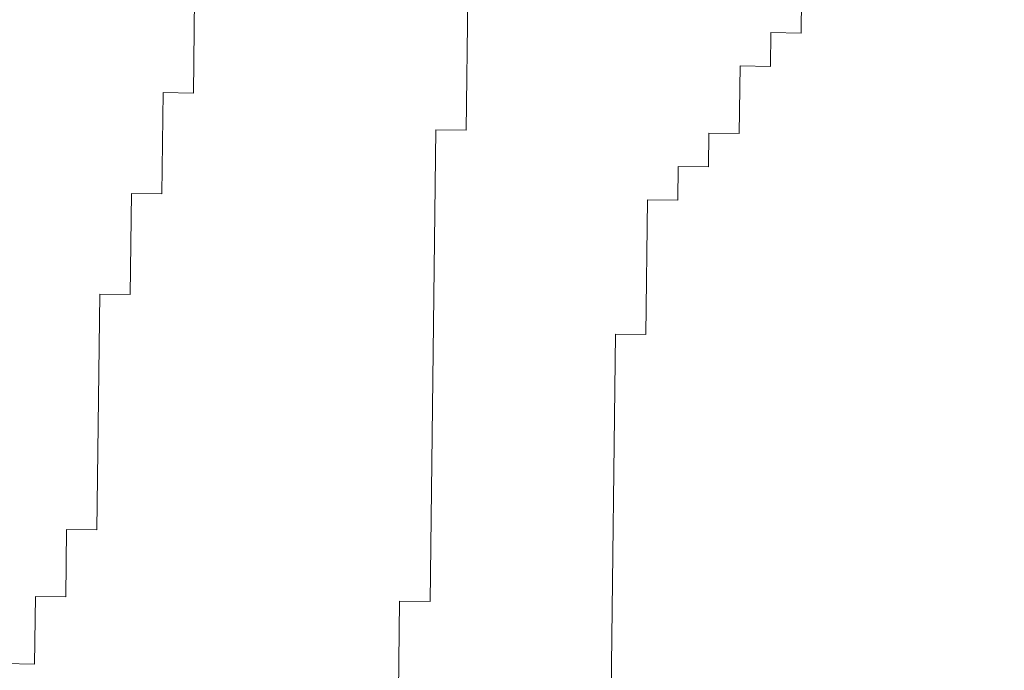
# Model space of a CAD drawing. Units: inches. Extents: x -466983 to 1020, y 324 to 318697.
# Tile 70 of 97: x 643.839 to 647.874, y 942.656 to 945.322. Entities that reach past the tile are written whole.
import ezdxf

# ---------------------------------------------------------------- set-up
doc = ezdxf.new("R2010")
doc.units = ezdxf.units.IN
doc.header["$MEASUREMENT"] = 0
doc.layers.add('A-FLOR-PATT', color=252, linetype='Continuous', lineweight=13)
doc.layers.add('A-FURN', color=8, linetype='Continuous', lineweight=18)

# ---------------------------------------------------------------- blocks, each defined once
blk = doc.blocks.new('L Shaped Sofa')
at = {"ltscale": 2}
for p, q in [((2414.2017, 741.2953), (2414.2417, 744.5701)), ((2415.8142, 743.2912), (2415.8234, 744.0469)), ((2418.5362, 743.2579), (2418.5424, 743.7617)), ((2418.5424, 743.7617), (2418.7692, 743.759)), ((2415.5443, 739.7672), (2415.5874, 743.294)), ((2415.5874, 743.294), (2415.8142, 743.2912)), ((2418.3033, 742.7569), (2418.3094, 743.2607)), ((2418.3094, 743.2607), (2418.5362, 743.2579)), ((2418.0549, 740.9963), (2418.0764, 742.7596)), ((2418.0764, 742.7596), (2418.3033, 742.7569)), ((2413.9626, 740.2904), (2413.9749, 741.2981)), ((2413.9749, 741.2981), (2414.2017, 741.2953)), ((2417.8188, 740.2433), (2417.828, 740.999)), ((2417.828, 740.999), (2418.0549, 740.9963)), ((2413.7327, 740.0413), (2413.7357, 740.2932)), ((2413.7357, 740.2932), (2413.9626, 740.2904)), ((2417.5827, 739.4903), (2417.592, 740.2461)), ((2417.592, 740.2461), (2417.8188, 740.2433)), ((2413.5028, 739.7921), (2413.5058, 740.044)), ((2413.5058, 740.044), (2413.7327, 740.0413)), ((2413.2698, 739.2911), (2413.2759, 739.7949)), ((2413.2759, 739.7949), (2413.5028, 739.7921)), ((2415.2897, 737.5028), (2415.3174, 739.77)), ((2415.3174, 739.77), (2415.5443, 739.7672)), ((2417.3467, 738.7374), (2417.3559, 739.4931)), ((2417.3559, 739.4931), (2417.5827, 739.4903)), ((2413.0398, 739.0419), (2413.0429, 739.2938)), ((2413.0429, 739.2938), (2413.2698, 739.2911)), ((2412.8069, 738.5409), (2412.813, 739.0447)), ((2412.813, 739.0447), (2413.0398, 739.0419))]:
    blk.add_line(p, q, dxfattribs=at)

msp = doc.modelspace()

# ---------------------------------------------------------------- hatches: boundary and pattern name
at = {"layer": 'A-FLOR-PATT', "transparency": 33554572}
h = msp.add_hatch(dxfattribs=at)
h.set_pattern_fill('ANSI37', color=256, scale=30)
h.set_pattern_definition([(45, (-1212.4137, -290.035), (-2.6516504, 2.6516504), []), (135, (-1212.4137, -290.035), (-2.6516504, -2.6516504), [])])
h.paths.add_polyline_path([(901.8057, 1075.9377), (900.6144, 1075.9377), (900.6144, 1065.3856), (899.391, 1065.3856), (898.0911, 1065.3856), (892.8356, 1058.7098, -0.258377), (892.1875, 1058.3509), (879.9848, 1058.3509, -0.20177), (879.4382, 1058.5808), (874.0812, 1065.3856), (872.7813, 1065.3856), (871.5579, 1065.3856), (871.5579, 1075.9377), (813.8057, 1075.9377), (813.8057, 1044.7922), (832.3947, 1044.7922, -0.394795), (848.6602, 1028.5356), (848.6602, 1009.9377), (901.8057, 1009.9377), (901.8057, 1015.9377), (901.3057, 1015.9377), (871.3057, 1015.9377), (871.3057, 1017.2502), (871.3344, 1017.2502, -0.401453), (901.3057, 1045.9377), (901.8057, 1045.9377)])
edge = h.paths.add_edge_path(flags=16)
edge.add_line((847.7731, 1068.9486), (847.7731, 1073.7088))
edge.add_arc((849.2269, 1073.7088), 1.4538, 90, 180, ccw=False)
edge.add_line((849.2269, 1075.1627), (864.4921, 1075.1627))
edge.add_arc((864.4921, 1073.7088), 1.4538, 0, 90, ccw=False)
edge.add_line((865.9459, 1073.7088), (865.9459, 1069.0035))
edge.add_arc((832.6447, 1068.9761), 33.3012, -20.61234, 0.04725, ccw=False)
edge.add_ellipse((856.8595, 1058.48), major_axis=(0, 10.2131), ratio=0.6859192, start_angle=100.00884, end_angle=259.99116, ccw=False)
edge.add_arc((881.0742, 1068.9761), 33.3012, 180.04725, 200.61234, ccw=False)
h.paths.add_polyline_path([(853.1456, 1066.4815), (853.1456, 1066.4534), (853.1463, 1066.4534, 0.433107), (852.9166, 1066.6849), (852.9166, 1066.4534), (853.1456, 1066.4534), (853.1456, 1066.4815), (853.088, 1066.6122, 0.697939), (852.6995, 1066.4534), (852.7003, 1066.4534), (852.7003, 1066.4815), (852.9166, 1067.0012), (852.9166, 1066.6849, -0.396254)], flags=0)
h.paths.add_polyline_path([(861.0187, 1066.4815), (861.0187, 1066.4534), (861.0194, 1066.4534, 0.416404), (860.8024, 1066.6849), (860.8024, 1066.4534), (861.0187, 1066.4534), (861.0187, 1066.4815), (860.9672, 1066.6053, 0.713344), (860.5726, 1066.4534), (860.5734, 1066.4534), (860.5734, 1066.4815), (860.8024, 1067.0012), (860.8024, 1066.6849, -0.379973)], flags=0)
edge = h.paths.add_edge_path(flags=0)
edge.add_spline(control_points=[(861.1298, 1065.7855), (861.4661, 1065.2478), (861.6134, 1065.0161), (861.9833, 1064.3736), (862.1924, 1063.9443), (862.5614, 1063.0391), (862.7212, 1062.5633), (862.9865, 1061.5781), (863.092, 1061.0689), (863.2452, 1060.031), (863.293, 1059.5025), (863.3295, 1058.4409), (863.3181, 1057.9078), (863.2366, 1056.8518), (863.1664, 1056.3289), (862.9695, 1055.308), (862.8427, 1054.8099), (862.5365, 1053.8522), (862.3571, 1053.3927), (861.9514, 1052.5249), (861.7251, 1052.1166), (861.233, 1051.3622), (860.9672, 1051.0162), (860.4048, 1050.3949), (860.1082, 1050.1197), (859.4937, 1049.6461), (859.1758, 1049.4476), (858.5276, 1049.1299), (858.1973, 1049.0107), (857.5315, 1048.8518), (857.1959, 1048.8121), (856.5249, 1048.812), (856.1894, 1048.8515), (855.5236, 1049.0101), (855.1933, 1049.1291), (854.545, 1049.4465), (854.2271, 1049.6449), (853.6124, 1050.1183), (853.3158, 1050.3933), (852.7533, 1051.0143), (852.4874, 1051.3602), (851.9952, 1052.1144), (851.7688, 1052.5225), (851.3629, 1053.3902), (851.1834, 1053.8496), (850.877, 1054.8071), (850.7501, 1055.3051), (850.553, 1056.326), (850.4827, 1056.8488), (850.401, 1057.9048), (850.3895, 1058.4379), (850.4257, 1059.4995), (850.4734, 1060.0281), (850.6265, 1061.066), (850.7318, 1061.5753), (850.9969, 1062.5605), (851.1567, 1063.0365), (851.5254, 1063.9418), (851.7345, 1064.3712), (852.1056, 1065.0164), (852.2544, 1065.2503), (852.6082, 1065.7335)], knot_values=[3.915332, 3.915332, 3.915332, 3.915332, 4.013468, 4.013468, 4.175532, 4.175532, 4.337596, 4.337596, 4.49966, 4.49966, 4.661724, 4.661724, 4.823788, 4.823788, 4.985852, 4.985852, 5.147916, 5.147916, 5.30998, 5.30998, 5.472044, 5.472044, 5.634109, 5.634109, 5.796173, 5.796173, 5.958237, 5.958237, 6.120301, 6.120301, 6.282365, 6.282365, 6.444429, 6.444429, 6.606493, 6.606493, 6.768557, 6.768557, 6.930621, 6.930621, 7.092685, 7.092685, 7.254749, 7.254749, 7.416813, 7.416813, 7.578878, 7.578878, 7.740942, 7.740942, 7.903006, 7.903006, 8.06507, 8.06507, 8.227134, 8.227134, 8.389198, 8.389198, 8.551262, 8.551262, 8.65037, 8.65037, 8.65037, 8.65037], degree=3, periodic=0)
edge.add_line((852.6421, 1065.7855), (861.1298, 1065.7855))
edge = h.paths.add_edge_path(flags=0)
edge.add_ellipse((856.8496, 1057.7432), major_axis=(0, 7.7921), ratio=0.687861, start_angle=0, end_angle=360)
h.paths.add_polyline_path([(848.8634, 1069.3891), (848.8634, 1073.9605, -0.414214), (849.9538, 1075.0508), (863.7652, 1075.0508, -0.414214), (864.8555, 1073.9605), (864.8555, 1069.3891, -0.388936), (864.5237, 1069.027, -0.043561), (849.1953, 1069.027, -0.388936)], flags=0)
h.paths.add_polyline_path([(853.1006, 1068.1122, -1), (852.6775, 1068.1122, -1)], flags=0)
edge = h.paths.add_edge_path(flags=0)
edge.add_ellipse((856.8595, 1057.3378), major_axis=(0, 2.207), ratio=0.657164, start_angle=0, end_angle=360)
h.paths.add_polyline_path([(861.0415, 1068.1122, -1), (860.6184, 1068.1122, -1)], flags=0)
edge = h.paths.add_edge_path()
edge.add_line((573.9537, 1057.3412), (573.9537, 1075.9377))
edge.add_line((573.9537, 1075.9377), (558.7308, 1075.9377))
edge.add_line((558.7308, 1075.9377), (558.7308, 1065.3856))
edge.add_line((558.7308, 1065.3856), (557.5074, 1065.3856))
edge.add_line((557.5074, 1065.3856), (556.2075, 1065.3856))
edge.add_line((556.2075, 1065.3856), (550.952, 1058.7098))
edge.add_arc((550.3039, 1059.1155), 0.7646, 270, 327.9483, ccw=False)
edge.add_line((550.3039, 1058.3509), (538.1012, 1058.3509))
edge.add_arc((538.1012, 1059.1155), 0.7646, 224.3704, 270, ccw=False)
edge.add_line((537.5546, 1058.5808), (532.1976, 1065.3856))
edge.add_line((532.1976, 1065.3856), (530.8977, 1065.3856))
edge.add_line((530.8977, 1065.3856), (529.6743, 1065.3856))
edge.add_line((529.6743, 1065.3856), (529.6743, 1075.9377))
edge.add_line((529.6743, 1075.9377), (520.8057, 1075.9377))
edge.add_line((520.8057, 1075.9377), (520.8057, 1045.9377))
edge.add_line((520.8057, 1045.9377), (521.3057, 1045.9377))
edge.add_arc((521.3057, 1015.9377), 30, 2.50749, 90, ccw=False)
edge.add_line((551.277, 1017.2502), (551.3057, 1017.2502))
edge.add_line((551.3057, 1017.2502), (551.3057, 1015.9377))
edge.add_line((551.3057, 1015.9377), (520.8057, 1015.9377))
edge.add_line((520.8057, 1015.9377), (520.8057, 1009.9377))
edge.add_line((520.8057, 1009.9377), (559.1913, 1010.4022))
edge.add_arc((559.1913, 1011.856), 1.4538, 180, 270, ccw=False)
edge.add_line((557.7375, 1011.856), (557.7375, 1016.5613))
edge.add_arc((591.0386, 1016.5888), 33.3012, 159.38766, 180.04725, ccw=False)
edge.add_ellipse((566.8239, 1027.0848), major_axis=(0, 10.2131), ratio=0.6859192, start_angle=280.00884, end_angle=439.99116, ccw=False)
edge.add_arc((542.6091, 1016.5888), 33.3012, 0.04725, 20.61234, ccw=False)
edge.add_line((575.9103, 1016.6162), (575.9103, 1011.856))
edge.add_arc((574.4565, 1011.856), 1.4538, -90, 0, ccw=False)
edge.add_line((574.4565, 1010.4022), (608.8057, 1009.9377))
edge.add_line((608.8057, 1009.9377), (608.8057, 1041.0857))
edge.add_line((608.8057, 1041.0857), (590.2179, 1041.0857))
edge.add_arc((590.775, 1057.9074), 16.8309, 181.92775, 268.10321, ccw=False)
edge = h.paths.add_edge_path()
edge.add_ellipse((494.2443, 583.6204), major_axis=(0, 10.2131), ratio=0.6859192, start_angle=280.00884, end_angle=439.99116, ccw=False)
edge.add_arc((470.0296, 573.1243), 33.3012, 0.04725, 20.61234, ccw=False)
edge.add_line((503.3307, 573.1518), (503.3307, 568.3916))
edge.add_arc((501.8769, 568.3916), 1.4538, -90, 0, ccw=False)
edge.add_line((501.8769, 566.9377), (539.8057, 566.9377))
edge.add_line((539.8057, 566.9377), (539.8057, 572.9377))
edge.add_line((539.8057, 572.9377), (539.3057, 572.9377))
edge.add_line((539.3057, 572.9377), (509.3057, 572.9377))
edge.add_line((509.3057, 572.9377), (509.3057, 574.2502))
edge.add_line((509.3057, 574.2502), (509.3344, 574.2502))
edge.add_arc((539.3057, 572.9377), 30, 90, 177.49251, ccw=False)
edge.add_line((539.3057, 602.9377), (539.8057, 602.9377))
edge.add_line((539.8057, 602.9377), (539.8057, 626.9377))
edge.add_line((539.8057, 626.9377), (531.7718, 626.9377))
edge.add_line((531.7718, 626.9377), (531.7718, 616.3856))
edge.add_line((531.7718, 616.3856), (530.5484, 616.3856))
edge.add_line((530.5484, 616.3856), (529.2485, 616.3856))
edge.add_line((529.2485, 616.3856), (523.7105, 609.3509))
edge.add_line((523.7105, 609.3509), (510.7766, 609.3509))
edge.add_line((510.7766, 609.3509), (505.2386, 616.3856))
edge.add_line((505.2386, 616.3856), (503.9387, 616.3856))
edge.add_line((503.9387, 616.3856), (502.7153, 616.3856))
edge.add_line((502.7153, 616.3856), (502.7153, 626.9377))
edge.add_line((502.7153, 626.9377), (481.6983, 626.9377))
edge.add_line((481.6983, 626.9377), (481.6983, 610.995))
edge.add_arc((467.2703, 611.4728), 14.4359, 271.92775, 358.10321, ccw=False)
edge.add_line((467.7559, 597.0451), (451.8057, 597.0451))
edge.add_line((451.8057, 597.0451), (451.8057, 584.4035))
edge.add_line((451.8057, 584.4035), (451.8057, 566.9377))
edge.add_line((451.8057, 566.9377), (486.6117, 566.9377))
edge.add_arc((486.6117, 568.3916), 1.4538, 180, 270, ccw=False)
edge.add_line((485.1579, 568.3916), (485.1579, 573.0969))
edge.add_arc((518.4591, 573.1243), 33.3012, 159.38766, 180.04725, ccw=False)
h.paths.add_polyline_path([(836.2609, 1020.7328), (879.8898, 1020.7328), (879.8898, 1039.3902), (836.2609, 1039.3902)], flags=25)
h.paths.add_polyline_path([(549.9851, 1036.7492), (593.614, 1036.7492), (593.614, 1055.4065), (549.9851, 1055.4065)], flags=24)
h.paths.add_polyline_path([(475.123, 595.5959), (518.752, 595.5959), (518.752, 614.2532), (475.123, 614.2532)], flags=24)
h = msp.add_hatch(dxfattribs=at)
h.set_pattern_fill('ANSI37', color=256, scale=20)
h.set_pattern_definition([(45, (-1212.4137, -290.035), (-1.767767, 1.767767), []), (135, (-1212.4137, -290.035), (-1.767767, -1.767767), [])])
h.paths.add_polyline_path([(809.8057, 870.9377), (809.8057, 888.1519), (806.9985, 888.1519), (802.6624, 888.1519), (789.3832, 888.1519), (786.2846, 888.1519, -0.414214), (785.4991, 888.9374), (785.4991, 900.1959), (785.4991, 908.4696, -0.414214), (786.8082, 909.7787, -0.414214), (785.4991, 911.0878), (785.4991, 929.1015, -0.414214), (786.8082, 930.4106, -0.414214), (785.4991, 931.7197), (785.4991, 931.9039, -0.414214), (784.19, 930.5948), (766.7223, 930.5948, -0.412359), (765.4132, 931.8956, -0.413741), (764.1145, 930.5782), (744.5781, 930.422, -0.416556), (743.7864, 931.2075), (743.7864, 933.5153), (742.2154, 933.5153), (742.2154, 952.024, -0.001344), (743.7864, 952.1998), (743.7864, 953.9377), (678.5915, 953.9377), (678.5915, 951.1305), (678.5915, 946.7945), (678.5915, 933.5153), (678.5915, 930.4166, -0.414214), (677.806, 929.6312), (666.5475, 929.6312), (658.2738, 929.6312, -0.414214), (656.9647, 930.9403, -0.414214), (655.6556, 929.6312), (637.6419, 929.6312, -0.414214), (636.3328, 930.9403, -0.414214), (635.0237, 929.6312), (634.8395, 929.6312, -0.414214), (636.1486, 928.322), (636.1486, 910.8544, -0.412359), (634.8478, 909.5452, -0.413741), (636.1653, 908.2466), (636.3214, 888.7102, -0.416556), (635.5359, 887.9184), (633.2281, 887.9184), (633.2281, 886.3475), (614.7194, 886.3475, -0.001344), (614.5436, 887.9184), (612.8057, 887.9184), (612.8057, 834.9377), (612.8057, 752.9377), (612.8057, 748.9377), (612.8057, 697.9377), (654.8057, 697.9377), (654.8057, 701.9377), (715.8057, 701.9377), (715.8057, 737.4353), (774.2918, 737.4353), (774.2918, 795.9377), (809.8057, 795.9377)])
h.paths.add_polyline_path([(679.2761, 849.5757, 0.102523), (682.1475, 849.2608, -0.080461), (694.5428, 849.7725, -0.283899), (694.4822, 849.0082, 0.136605), (694.4068, 848.8103, -0.030441), (694.5428, 846.8929), (694.5428, 842.6198), (694.5428, 838.3466, -0.028219), (694.4246, 836.5684), (694.425, 836.5684, 0.196187), (694.4456, 836.2708, -0.302897), (694.5428, 835.467, -0.080461), (682.1475, 835.9787, 0.102523), (679.2761, 835.6638, -0.58611), (678.6457, 836.0169), (678.6457, 849.2227, -0.58611)], flags=16)
h.paths.add_polyline_path([(679.5173, 848.6515, 0.699597), (679.476, 848.6342, 1.20716), (679.1935, 848.7422, 0.010621)], flags=0)
h.paths.add_polyline_path([(679.4923, 836.5608, -0.013798), (679.9178, 836.6594, -0.071703), (682.8533, 837.1434, -0.165743), (682.1665, 839.1006), (682.1665, 842.6094), (682.1665, 846.0603, -0.240616), (683.4733, 848.6767, -0.068263), (693.9295, 849.0082), (693.7875, 848.7083), (693.7875, 849.0228, 0.067332), (683.4733, 848.6767, 0.240616), (682.1665, 846.0603), (682.1665, 842.6094), (682.1665, 839.1006, 0.23459), (683.461, 836.5513, 0.068093), (693.7875, 836.1955), (693.7875, 836.5104), (693.9296, 836.2102, -0.077215), (682.2421, 836.7815, 0.086627), (679.5283, 836.5701, -0.628402), (679.5029, 836.5735), (679.5029, 836.6071, 0.910458)], flags=0)
h.paths.add_polyline_path([(679.476, 848.6364), (679.2069, 848.647), (679.2069, 836.5718, 0.913566), (679.3645, 836.5861), (679.476, 836.5824)], flags=0)
h.paths.add_polyline_path([(679.2761, 829.8604, 0.102523), (682.1475, 829.5455, -0.080461), (694.5428, 830.0572, -0.283899), (694.4822, 829.2929, 0.136605), (694.4068, 829.095, -0.030441), (694.5428, 827.1776), (694.5428, 822.9045), (694.5428, 818.6314, -0.028219), (694.4246, 816.8531), (694.425, 816.8532, 0.196187), (694.4456, 816.5555, -0.302897), (694.5428, 815.7517, -0.080461), (682.1475, 816.2635, 0.102523), (679.2761, 815.9485, -0.58611), (678.6457, 816.3016), (678.6457, 829.5074, -0.58611)], flags=16)
h.paths.add_polyline_path([(679.5173, 828.9362, 0.699597), (679.476, 828.9189, 1.20716), (679.1935, 829.0269, 0.010621)], flags=0)
h.paths.add_polyline_path([(679.4923, 816.8456, -0.013798), (679.9178, 816.9441, -0.071703), (682.8533, 817.4281, -0.165743), (682.1665, 819.3853), (682.1665, 822.8941), (682.1665, 826.345, -0.240616), (683.4733, 828.9614, -0.068263), (693.9295, 829.2929), (693.7875, 828.9931), (693.7875, 829.3076, 0.067332), (683.4733, 828.9614, 0.240616), (682.1665, 826.345), (682.1665, 822.8941), (682.1665, 819.3853, 0.23459), (683.461, 816.836, 0.068093), (693.7875, 816.4802), (693.7875, 816.7952), (693.9296, 816.4949, -0.077215), (682.2421, 817.0662, 0.086627), (679.5283, 816.8549, -0.628402), (679.5029, 816.8582), (679.5029, 816.8918, 0.910458)], flags=0)
h.paths.add_polyline_path([(679.476, 828.9211), (679.2069, 828.9317), (679.2069, 816.8565, 0.913566), (679.3645, 816.8708), (679.476, 816.8671)], flags=0)
h.paths.add_polyline_path([(679.2761, 810.1451, 0.102523), (682.1475, 809.8302, -0.080461), (694.5428, 810.342, -0.3023), (694.4466, 809.5394, 0.10023), (694.4058, 809.3878, -0.03057), (694.5428, 807.4623), (694.5428, 803.1892), (694.5428, 798.9161, -0.03057), (694.4058, 796.9906, 0.10023), (694.4466, 796.839, -0.3023), (694.5428, 796.0365, -0.080461), (682.1475, 796.5482, 0.102523), (679.2761, 796.2333, -0.58611), (678.6457, 796.5863), (678.6457, 809.7921, -0.58611)], flags=16)
h.paths.add_polyline_path([(679.5173, 809.2417, 0.699597), (679.476, 809.2244, 1.20716), (679.1935, 809.3324, 0.010621)], flags=0)
h.paths.add_polyline_path([(679.4923, 797.151, -0.013798), (679.9178, 797.2496, -0.071703), (682.8533, 797.7336, -0.165743), (682.1665, 799.6908), (682.1665, 803.1996), (682.1665, 806.6505, -0.239349), (683.461, 809.2577, -0.072465), (694.4468, 809.5405, 0.197932), (694.425, 809.2405), (693.7875, 809.2985), (693.7875, 809.6135, 0.068093), (683.461, 809.2577, 0.239349), (682.1665, 806.6505), (682.1665, 803.1996), (682.1665, 799.6908, 0.235854), (683.4733, 797.1323, 0.067332), (693.7875, 796.7861), (693.7875, 797.1006), (694.425, 797.1586, 0.197932), (694.4468, 796.8586, -0.080419), (682.1557, 797.3795, 0.083867), (679.5283, 797.1603, -0.628402), (679.5029, 797.1637), (679.5029, 797.1973, 0.910458)], flags=0)
h.paths.add_polyline_path([(679.2069, 809.2372), (679.2069, 797.162, 0.913566), (679.3645, 797.1763), (679.476, 797.1726), (679.476, 809.2266)], flags=0)
h.paths.add_polyline_path([(695.3643, 853.2989), (728.2231, 853.2989), (728.2231, 771.1519), (695.3643, 771.1519)], flags=16)
h.paths.add_polyline_path([(696.0215, 852.6417), (727.5659, 852.6417), (727.5659, 771.809), (696.0215, 771.809)], flags=0)
h.paths.add_polyline_path([(679.2761, 788.7869, 0.102523), (682.1475, 788.472, -0.080461), (694.5428, 788.9837, -0.3023), (694.4466, 788.1812, 0.10023), (694.4058, 788.0296, -0.03057), (694.5428, 786.1041), (694.5428, 781.831), (694.5428, 777.5578, -0.03057), (694.4058, 775.6323, 0.10023), (694.4466, 775.4808, -0.3023), (694.5428, 774.6782, -0.080461), (682.1475, 775.19, 0.102523), (679.2761, 774.875, -0.58611), (678.6457, 775.2281), (678.6457, 788.4339, -0.58611)], flags=16)
h.paths.add_polyline_path([(679.5173, 787.8834, 0.699597), (679.476, 787.8662, 1.20716), (679.1935, 787.9742, 0.010621)], flags=0)
h.paths.add_polyline_path([(679.4923, 775.7928, -0.013798), (679.9178, 775.8914, -0.071703), (682.8533, 776.3753, -0.165743), (682.1665, 778.3325), (682.1665, 781.8414), (682.1665, 785.2922, -0.239349), (683.461, 787.8995, -0.072465), (694.4468, 788.1823, 0.197932), (694.425, 787.8823), (693.7875, 787.9403), (693.7875, 788.2553, 0.068093), (683.461, 787.8995, 0.239349), (682.1665, 785.2922), (682.1665, 781.8414), (682.1665, 778.3325, 0.235854), (683.4733, 775.7741, 0.067332), (693.7875, 775.4279), (693.7875, 775.7424), (694.425, 775.8004, 0.197932), (694.4468, 775.5004, -0.080419), (682.1557, 776.0212, 0.083867), (679.5283, 775.8021, -0.628402), (679.5029, 775.8054), (679.5029, 775.8391, 0.910458)], flags=0)
h.paths.add_polyline_path([(679.2069, 787.8789), (679.2069, 775.8038, 0.913566), (679.3645, 775.818), (679.476, 775.8144), (679.476, 787.8684)], flags=0)
h.paths.add_polyline_path([(704.641, 854.1204, -0.080461), (705.1527, 866.5157, 0.102523), (704.8378, 869.3871, -0.58611), (705.1908, 870.0174), (718.3966, 870.0174, -0.58611), (718.7496, 869.3871, 0.102523), (718.4347, 866.5157, -0.080461), (718.9465, 854.1204, -0.3023), (718.1439, 854.2166, 0.10023), (717.9924, 854.2574, -0.03057), (716.0668, 854.1204), (711.7937, 854.1204), (707.5206, 854.1204, -0.03057), (705.5951, 854.2574, 0.10023), (705.4435, 854.2166, -0.3023)], flags=16)
h.paths.add_polyline_path([(717.8462, 869.1459, 0.699597), (717.8289, 869.1872, 1.20716), (717.9369, 869.4697, 0.010621)], flags=0)
h.paths.add_polyline_path([(705.4631, 854.2164, -0.080419), (705.984, 866.5074, 0.083867), (705.7648, 869.1349, -0.628402), (705.7682, 869.1603), (705.8018, 869.1603, 0.910458), (705.7555, 869.1709, -0.013798), (705.8541, 868.7454, -0.071703), (706.3381, 865.8099, -0.165743), (708.2953, 866.4967), (711.8041, 866.4967), (715.255, 866.4967, -0.239349), (717.8622, 865.2022, -0.072465), (718.145, 854.2164, 0.197932), (717.845, 854.2382), (717.903, 854.8757), (718.218, 854.8757, 0.068093), (717.8622, 865.2022, 0.239349), (715.255, 866.4967), (711.8041, 866.4967), (708.2953, 866.4967, 0.235854), (705.7368, 865.1898, 0.067332), (705.3906, 854.8757), (705.7051, 854.8757), (705.7631, 854.2382, 0.197932)], flags=16)
h.paths.add_polyline_path([(705.7665, 869.4563, 0.913566), (705.7808, 869.2987), (705.7771, 869.1872), (717.8311, 869.1872), (717.8417, 869.4563)], flags=0)
h.paths.add_polyline_path([(729.0446, 842.6198), (729.0446, 846.8929, -0.03057), (729.1817, 848.8184, 0.10023), (729.1408, 848.9699, -0.3023), (729.0446, 849.7725, -0.080461), (741.4399, 849.2608, 0.102523), (744.3113, 849.5757, -0.58611), (744.9417, 849.2227), (744.9417, 836.0169, -0.58611), (744.3113, 835.6638, 0.102523), (741.4399, 835.9787, -0.080461), (729.0446, 835.467, -0.3023), (729.1408, 836.2696, 0.10023), (729.1817, 836.4211, -0.03057), (729.0446, 838.3466)], flags=16)
h.paths.add_polyline_path([(744.1115, 836.5846, 1.20716), (744.3939, 836.4766, 0.010621), (744.0701, 836.5673, 0.699597)], flags=0)
h.paths.add_polyline_path([(729.1407, 836.2684, 0.197932), (729.1624, 836.5684), (729.7999, 836.5104), (729.7999, 836.1955, 0.068093), (740.1264, 836.5513, 0.239349), (741.4209, 839.1585), (741.4209, 842.6094), (741.4209, 846.1182, 0.235854), (740.1141, 848.6767, 0.067332), (729.7999, 849.0228), (729.7999, 848.7083), (729.1624, 848.6503, 0.197932), (729.1407, 848.9504, -0.080419), (741.4317, 848.4295, 0.083867), (744.0591, 848.6486, -0.628402), (744.0845, 848.6453), (744.0845, 848.6117, 0.910458), (744.0951, 848.6579, -0.013798), (743.6696, 848.5594, -0.071703), (740.7341, 848.0754, -0.165743), (741.4209, 846.1182), (741.4209, 842.6094), (741.4209, 839.1585, -0.239349), (740.1264, 836.5513, -0.072465)], flags=0)
h.paths.add_polyline_path([(729.0446, 830.0572, -0.080461), (741.4399, 829.5455, 0.102523), (744.3113, 829.8604, -0.58611), (744.9417, 829.5074), (744.9417, 816.3016, -0.58611), (744.3113, 815.9485, 0.102523), (741.4399, 816.2635, -0.080461), (729.0446, 815.7517, -0.3023), (729.1408, 816.5543, 0.10023), (729.1817, 816.7058, -0.03057), (729.0446, 818.6314), (729.0446, 822.9045), (729.0446, 827.1776, -0.03057), (729.1817, 829.1031, 0.10023), (729.1408, 829.2547, -0.3023)], flags=16)
h.paths.add_polyline_path([(744.1115, 816.8693, 1.20716), (744.3939, 816.7613, 0.010621), (744.0701, 816.852, 0.699597)], flags=0)
h.paths.add_polyline_path([(729.1407, 829.2351, -0.080419), (741.4317, 828.7142, 0.083867), (744.0591, 828.9334, -0.628402), (744.0845, 828.93), (744.0845, 828.8964, 0.910458), (744.0951, 828.9427, -0.013798), (743.6696, 828.8441, -0.071703), (740.7341, 828.3601, -0.165743), (741.4209, 826.4029), (741.4209, 822.8941), (741.4209, 819.4432, -0.239349), (740.1264, 816.836, -0.072465), (729.1407, 816.5531, 0.197932), (729.1624, 816.8532), (729.7999, 816.7952), (729.7999, 816.4802, 0.068093), (740.1264, 816.836, 0.239349), (741.4209, 819.4432), (741.4209, 822.8941), (741.4209, 826.4029, 0.235854), (740.1141, 828.9614, 0.067332), (729.7999, 829.3076), (729.7999, 828.9931), (729.1624, 828.9351, 0.197932)], flags=16)
h.paths.add_polyline_path([(729.0446, 810.342, -0.080461), (741.4399, 809.8302, 0.102523), (744.3113, 810.1451, -0.58611), (744.9417, 809.7921), (744.9417, 796.5863, -0.58611), (744.3113, 796.2333, 0.102523), (741.4399, 796.5482, -0.080461), (729.0446, 796.0365, -0.283899), (729.1052, 796.8007, 0.136605), (729.1806, 796.9987, -0.030441), (729.0446, 798.9161), (729.0446, 803.1892), (729.0446, 807.4623, -0.028219), (729.1628, 809.2406), (729.1624, 809.2405, 0.196187), (729.1418, 809.5382, -0.302897)], flags=16)
h.paths.add_polyline_path([(744.1115, 797.1748, 1.20716), (744.3939, 797.0668, 0.010621), (744.0701, 797.1575, 0.699597)], flags=0)
h.paths.add_polyline_path([(741.3453, 809.0275, 0.086627), (744.0591, 809.2388, -0.628402), (744.0845, 809.2355), (744.0845, 809.2019, 0.910458), (744.0951, 809.2481, -0.013798), (743.6696, 809.1496, -0.071703), (740.7341, 808.6656, -0.165743), (741.4209, 806.7084), (741.4209, 803.1996), (741.4209, 799.7487, -0.240616), (740.1141, 797.1323, -0.068263), (729.658, 796.8008), (729.7999, 797.1006), (729.7999, 796.7861, 0.067332), (740.1141, 797.1323, 0.240616), (741.4209, 799.7487), (741.4209, 803.1996), (741.4209, 806.7084, 0.23459), (740.1264, 809.2577, 0.068093), (729.7999, 809.6135), (729.7999, 809.2985), (729.6578, 809.5988, -0.077215)], flags=0)
h.paths.add_polyline_path([(704.641, 770.3304, -0.283899), (705.4053, 770.2697, 0.136605), (705.6032, 770.1944, -0.030441), (707.5206, 770.3304), (711.7937, 770.3304), (716.0668, 770.3304, -0.028219), (717.8451, 770.2122), (717.845, 770.2126, 0.196187), (718.1427, 770.2331, -0.302897), (718.9465, 770.3304, -0.080461), (718.4347, 757.9351, 0.102523), (718.7496, 755.0637, -0.58611), (718.3966, 754.4333), (705.1908, 754.4333, -0.58611), (704.8378, 755.0637, 0.102523), (705.1527, 757.9351, -0.080461)], flags=16)
h.paths.add_polyline_path([(705.762, 755.3048, 0.699597), (705.7793, 755.2635, 1.20716), (705.6713, 754.9811, 0.010621)], flags=0)
h.paths.add_polyline_path([(705.4053, 769.717), (705.7051, 769.5751), (705.3906, 769.5751, 0.067332), (705.7368, 759.2609, 0.240616), (708.3532, 757.954), (711.8041, 757.954), (715.3129, 757.954, 0.23459), (717.8622, 759.2485, 0.068093), (718.218, 769.5751), (717.903, 769.5751), (718.2033, 769.7172, -0.077215), (717.632, 758.0297, 0.086627), (717.8433, 755.3159, -0.628402), (717.84, 755.2904), (717.8064, 755.2904, 0.910458), (717.8526, 755.2799, -0.013798), (717.7541, 755.7053, -0.071703), (717.2701, 758.6409, -0.165743), (715.3129, 757.954), (711.8041, 757.954), (708.3532, 757.954, -0.240616), (705.7368, 759.2609, -0.068263)], flags=0)
h.paths.add_polyline_path([(729.0446, 788.9837, -0.080461), (741.4399, 788.472, 0.102523), (744.3113, 788.7869, -0.58611), (744.9417, 788.4339), (744.9417, 775.2281, -0.58611), (744.3113, 774.875, 0.102523), (741.4399, 775.19, -0.080461), (729.0446, 774.6782, -0.283899), (729.1052, 775.4425, 0.136605), (729.1806, 775.6405, -0.030441), (729.0446, 777.5578), (729.0446, 781.831), (729.0446, 786.1041, -0.028219), (729.1628, 787.8823), (729.1624, 787.8823, 0.196187), (729.1418, 788.1799, -0.302897)], flags=16)
h.paths.add_polyline_path([(744.1115, 775.8165, 1.20716), (744.3939, 775.7086, 0.010621), (744.0701, 775.7993, 0.699597)], flags=0)
h.paths.add_polyline_path([(741.3453, 787.6692, 0.086627), (744.0591, 787.8806, -0.628402), (744.0845, 787.8773), (744.0845, 787.8437, 0.910458), (744.0951, 787.8899, -0.013798), (743.6696, 787.7913, -0.071703), (740.7341, 787.3074, -0.165743), (741.4209, 785.3502), (741.4209, 781.8414), (741.4209, 778.3905, -0.240616), (740.1141, 775.7741, -0.068263), (729.658, 775.4425), (729.7999, 775.7424), (729.7999, 775.4279, 0.067332), (740.1141, 775.7741, 0.240616), (741.4209, 778.3905), (741.4209, 781.8414), (741.4209, 785.3502, 0.23459), (740.1264, 787.8995, 0.068093), (729.7999, 788.2553), (729.7999, 787.9403), (729.6578, 788.2405, -0.077215)], flags=0)
h.paths.add_polyline_path([(744.1115, 848.6364), (744.1115, 836.5824), (744.3805, 836.5718), (744.3805, 848.647, 0.913566), (744.2229, 848.6327)], flags=0)
h.paths.add_polyline_path([(744.2229, 828.9174), (744.1115, 828.9211), (744.1115, 816.8671), (744.3805, 816.8565), (744.3805, 828.9317, 0.913566)], flags=0)
h.paths.add_polyline_path([(717.8311, 755.2635), (705.7771, 755.2635), (705.7665, 754.9945), (717.8417, 754.9945, 0.913566), (717.8274, 755.1521)], flags=0)
h.paths.add_polyline_path([(744.2229, 809.2229), (744.1115, 809.2266), (744.1115, 797.1726), (744.3805, 797.162), (744.3805, 809.2372, 0.913566)], flags=0)
h.paths.add_polyline_path([(744.1115, 787.8684), (744.1115, 775.8144), (744.3805, 775.8038), (744.3805, 787.8789, 0.913566), (744.2229, 787.8647)], flags=0)
h.paths.add_polyline_path([(678.8774, 877.1228), (737.6127, 877.1228), (737.6127, 899.5116), (678.8774, 899.5116)], flags=24)

# ---------------------------------------------------------------- linework, layer by layer
at = {"layer": 'A-FURN', "ltscale": 2}
for p, q in [((645.6838, 946.1129), (645.6686, 944.8699)), ((645.6838, 946.1129), (645.6686, 944.8699)), ((645.6838, 946.1129), (645.6686, 944.8699)), ((645.6838, 946.1129), (645.6686, 944.8699)), ((645.6838, 946.1129), (645.6686, 944.8699)), ((645.6838, 946.1129), (645.6686, 944.8699)), ((647.045, 945.5437), (647.0416, 945.2675)), ((647.045, 945.5437), (647.0416, 945.2675)), ((647.045, 945.5437), (647.0416, 945.2675)), ((647.045, 945.5437), (647.0416, 945.2675)), ((647.045, 945.5437), (647.0416, 945.2675)), ((647.045, 945.5437), (647.0416, 945.2675)), ((644.5562, 945.436), (644.5511, 945.0217)), ((644.5562, 945.436), (644.5511, 945.0217)), ((644.5562, 945.436), (644.5511, 945.0217)), ((644.5562, 945.436), (644.5511, 945.0217)), ((644.5562, 945.436), (644.5511, 945.0217)), ((644.5562, 945.436), (644.5511, 945.0217)), ((646.9173, 945.2691), (646.9156, 945.131)), ((646.9173, 945.2691), (646.9156, 945.131)), ((646.9173, 945.2691), (646.9156, 945.131)), ((646.9173, 945.2691), (646.9156, 945.131)), ((646.9173, 945.2691), (646.9156, 945.131)), ((646.9173, 945.2691), (646.9156, 945.131)), ((647.0416, 945.2675), (646.9173, 945.2691)), ((647.0416, 945.2675), (646.9173, 945.2691)), ((647.0416, 945.2675), (646.9173, 945.2691)), ((647.0416, 945.2675), (646.9173, 945.2691)), ((647.0416, 945.2675), (646.9173, 945.2691)), ((647.0416, 945.2675), (646.9173, 945.2691)), ((646.7912, 945.1325), (646.7878, 944.8563)), ((646.7912, 945.1325), (646.7878, 944.8563)), ((646.7912, 945.1325), (646.7878, 944.8563)), ((646.7912, 945.1325), (646.7878, 944.8563)), ((646.7912, 945.1325), (646.7878, 944.8563)), ((646.7912, 945.1325), (646.7878, 944.8563)), ((646.9156, 945.131), (646.7912, 945.1325)), ((646.9156, 945.131), (646.7912, 945.1325)), ((646.9156, 945.131), (646.7912, 945.1325)), ((646.9156, 945.131), (646.7912, 945.1325)), ((646.9156, 945.131), (646.7912, 945.1325)), ((646.9156, 945.131), (646.7912, 945.1325)), ((644.4268, 945.0232), (644.4217, 944.6089)), ((644.4268, 945.0232), (644.4217, 944.6089)), ((644.4268, 945.0232), (644.4217, 944.6089)), ((644.4268, 945.0232), (644.4217, 944.6089)), ((644.4268, 945.0232), (644.4217, 944.6089)), ((644.4268, 945.0232), (644.4217, 944.6089)), ((644.5511, 945.0217), (644.4268, 945.0232)), ((644.5511, 945.0217), (644.4268, 945.0232)), ((644.5511, 945.0217), (644.4268, 945.0232)), ((644.5511, 945.0217), (644.4268, 945.0232)), ((644.5511, 945.0217), (644.4268, 945.0232)), ((644.5511, 945.0217), (644.4268, 945.0232)), ((645.5443, 944.8715), (645.5207, 942.938)), ((645.5443, 944.8715), (645.5207, 942.938)), ((645.5443, 944.8715), (645.5207, 942.938)), ((645.5443, 944.8715), (645.5207, 942.938)), ((645.5443, 944.8715), (645.5207, 942.938)), ((645.5443, 944.8715), (645.5207, 942.938)), ((645.6686, 944.8699), (645.5443, 944.8715)), ((645.6686, 944.8699), (645.5443, 944.8715)), ((645.6686, 944.8699), (645.5443, 944.8715)), ((645.6686, 944.8699), (645.5443, 944.8715)), ((645.6686, 944.8699), (645.5443, 944.8715)), ((645.6686, 944.8699), (645.5443, 944.8715)), ((646.6635, 944.8578), (646.6618, 944.7197)), ((646.6635, 944.8578), (646.6618, 944.7197)), ((646.6635, 944.8578), (646.6618, 944.7197)), ((646.6635, 944.8578), (646.6618, 944.7197)), ((646.6635, 944.8578), (646.6618, 944.7197)), ((646.6635, 944.8578), (646.6618, 944.7197)), ((646.7878, 944.8563), (646.6635, 944.8578)), ((646.7878, 944.8563), (646.6635, 944.8578)), ((646.7878, 944.8563), (646.6635, 944.8578)), ((646.7878, 944.8563), (646.6635, 944.8578)), ((646.7878, 944.8563), (646.6635, 944.8578)), ((646.7878, 944.8563), (646.6635, 944.8578)), ((646.5374, 944.7212), (646.5358, 944.5831)), ((646.5374, 944.7212), (646.5358, 944.5831)), ((646.5374, 944.7212), (646.5358, 944.5831)), ((646.5374, 944.7212), (646.5358, 944.5831)), ((646.5374, 944.7212), (646.5358, 944.5831)), ((646.5374, 944.7212), (646.5358, 944.5831)), ((646.6618, 944.7197), (646.5374, 944.7212)), ((646.6618, 944.7197), (646.5374, 944.7212)), ((646.6618, 944.7197), (646.5374, 944.7212)), ((646.6618, 944.7197), (646.5374, 944.7212)), ((646.6618, 944.7197), (646.5374, 944.7212)), ((646.6618, 944.7197), (646.5374, 944.7212)), ((644.2974, 944.6105), (644.2923, 944.1962)), ((644.2974, 944.6105), (644.2923, 944.1962)), ((644.2974, 944.6105), (644.2923, 944.1962)), ((644.2974, 944.6105), (644.2923, 944.1962)), ((644.2974, 944.6105), (644.2923, 944.1962)), ((644.2974, 944.6105), (644.2923, 944.1962)), ((644.4217, 944.6089), (644.2974, 944.6105)), ((644.4217, 944.6089), (644.2974, 944.6105)), ((644.4217, 944.6089), (644.2974, 944.6105)), ((644.4217, 944.6089), (644.2974, 944.6105)), ((644.4217, 944.6089), (644.2974, 944.6105)), ((644.4217, 944.6089), (644.2974, 944.6105)), ((646.4114, 944.5846), (646.4047, 944.0322)), ((646.4114, 944.5846), (646.4047, 944.0322)), ((646.4114, 944.5846), (646.4047, 944.0322)), ((646.4114, 944.5846), (646.4047, 944.0322)), ((646.4114, 944.5846), (646.4047, 944.0322)), ((646.4114, 944.5846), (646.4047, 944.0322)), ((646.5358, 944.5831), (646.4114, 944.5846)), ((646.5358, 944.5831), (646.4114, 944.5846)), ((646.5358, 944.5831), (646.4114, 944.5846)), ((646.5358, 944.5831), (646.4114, 944.5846)), ((646.5358, 944.5831), (646.4114, 944.5846)), ((646.5358, 944.5831), (646.4114, 944.5846)), ((644.1679, 944.1977), (644.1561, 943.231)), ((644.1679, 944.1977), (644.1561, 943.231)), ((644.1679, 944.1977), (644.1561, 943.231)), ((644.1679, 944.1977), (644.1561, 943.231)), ((644.1679, 944.1977), (644.1561, 943.231)), ((644.1679, 944.1977), (644.1561, 943.231)), ((644.2923, 944.1962), (644.1679, 944.1977)), ((644.2923, 944.1962), (644.1679, 944.1977)), ((644.2923, 944.1962), (644.1679, 944.1977)), ((644.2923, 944.1962), (644.1679, 944.1977)), ((644.2923, 944.1962), (644.1679, 944.1977)), ((644.2923, 944.1962), (644.1679, 944.1977)), ((646.2803, 944.0337), (646.2584, 942.2384)), ((646.2803, 944.0337), (646.2584, 942.2384)), ((646.2803, 944.0337), (646.2584, 942.2384)), ((646.2803, 944.0337), (646.2584, 942.2384)), ((646.2803, 944.0337), (646.2584, 942.2384)), ((646.2803, 944.0337), (646.2584, 942.2384)), ((646.4047, 944.0322), (646.2803, 944.0337)), ((646.4047, 944.0322), (646.2803, 944.0337)), ((646.4047, 944.0322), (646.2803, 944.0337)), ((646.4047, 944.0322), (646.2803, 944.0337)), ((646.4047, 944.0322), (646.2803, 944.0337)), ((646.4047, 944.0322), (646.2803, 944.0337)), ((644.0318, 943.2325), (644.0284, 942.9563)), ((644.0318, 943.2325), (644.0284, 942.9563)), ((644.0318, 943.2325), (644.0284, 942.9563)), ((644.0318, 943.2325), (644.0284, 942.9563)), ((644.0318, 943.2325), (644.0284, 942.9563)), ((644.0318, 943.2325), (644.0284, 942.9563)), ((644.1561, 943.231), (644.0318, 943.2325)), ((644.1561, 943.231), (644.0318, 943.2325)), ((644.1561, 943.231), (644.0318, 943.2325)), ((644.1561, 943.231), (644.0318, 943.2325)), ((644.1561, 943.231), (644.0318, 943.2325)), ((644.1561, 943.231), (644.0318, 943.2325)), ((643.904, 942.9578), (643.9007, 942.6816)), ((643.904, 942.9578), (643.9007, 942.6816)), ((643.904, 942.9578), (643.9007, 942.6816)), ((643.904, 942.9578), (643.9007, 942.6816)), ((643.904, 942.9578), (643.9007, 942.6816)), ((643.904, 942.9578), (643.9007, 942.6816)), ((644.0284, 942.9563), (643.904, 942.9578)), ((644.0284, 942.9563), (643.904, 942.9578)), ((644.0284, 942.9563), (643.904, 942.9578)), ((644.0284, 942.9563), (643.904, 942.9578)), ((644.0284, 942.9563), (643.904, 942.9578)), ((644.0284, 942.9563), (643.904, 942.9578)), ((645.3963, 942.9396), (645.3913, 942.5253)), ((645.3963, 942.9396), (645.3913, 942.5253)), ((645.3963, 942.9396), (645.3913, 942.5253)), ((645.3963, 942.9396), (645.3913, 942.5253)), ((645.3963, 942.9396), (645.3913, 942.5253)), ((645.3963, 942.9396), (645.3913, 942.5253)), ((645.5207, 942.938), (645.3963, 942.9396)), ((645.5207, 942.938), (645.3963, 942.9396)), ((645.5207, 942.938), (645.3963, 942.9396)), ((645.5207, 942.938), (645.3963, 942.9396)), ((645.5207, 942.938), (645.3963, 942.9396)), ((645.5207, 942.938), (645.3963, 942.9396)), ((643.9007, 942.6816), (643.7763, 942.6831)), ((643.9007, 942.6816), (643.7763, 942.6831)), ((643.9007, 942.6816), (643.7763, 942.6831)), ((643.9007, 942.6816), (643.7763, 942.6831)), ((643.9007, 942.6816), (643.7763, 942.6831)), ((643.9007, 942.6816), (643.7763, 942.6831))]:
    msp.add_line(p, q, dxfattribs=at)

# ---------------------------------------------------------------- block references
at = {"layer": 'A-FURN', "xscale": 0.5482153745360612, "yscale": 0.5482153745360612, "zscale": 0.5482153745360612, "rotation": 180}
msp.add_blockref('L Shaped Sofa', (1969.7828, 1350.4232), dxfattribs=at)

doc.saveas('drawing.dxf')
